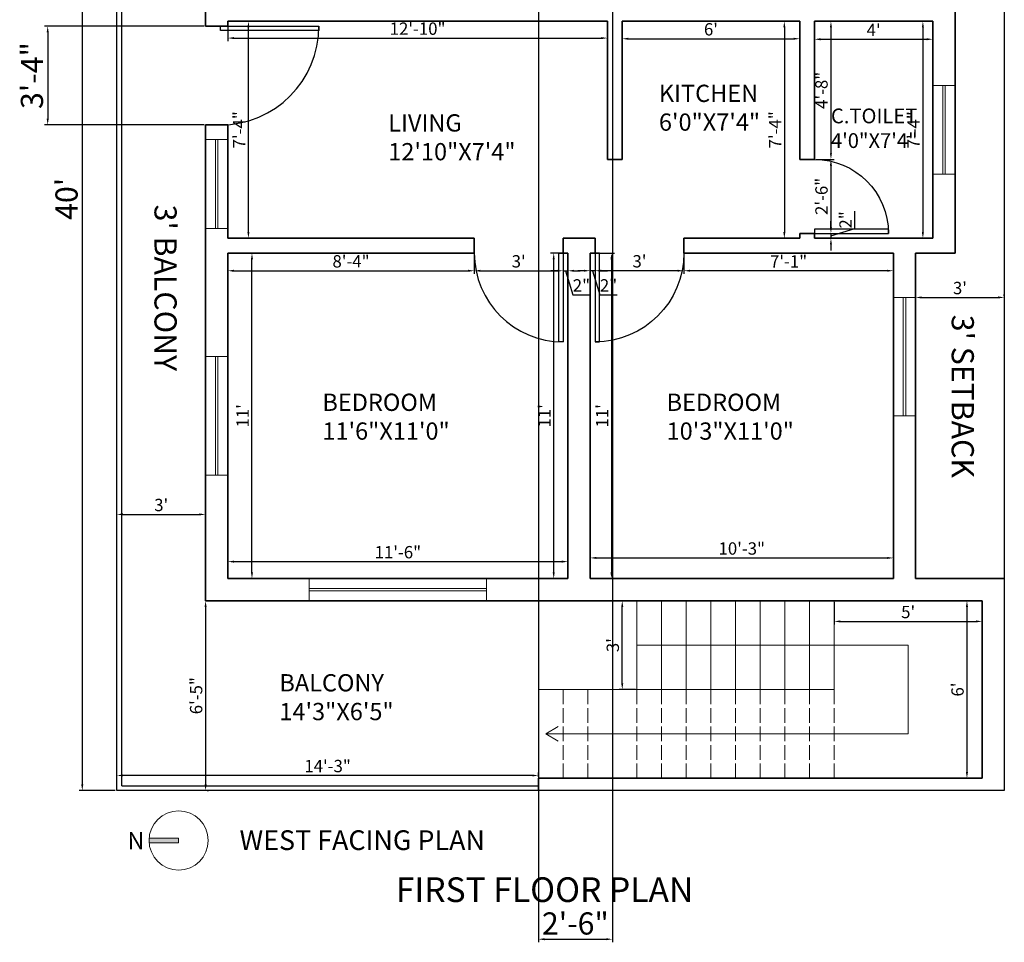
# Model space of a CAD drawing. Units: inches. Extents: x 2831 to 4250, y 1103 to 1797.
# Tile 14 of 15: x 3821 to 4220, y 1181 to 1555. Entities that reach past the tile are written whole.
import ezdxf

# ---------------------------------------------------------------- set-up
doc = ezdxf.new("R2010")
doc.units = ezdxf.units.IN
doc.linetypes.add('ACAD_ISO02W100', pattern=[15, 12, -3])
for name, color, linetype, lineweight in [('A-ANNO-DIMS', 2, 'Continuous', 18), ('A-ANNO-SYMB', 7, 'Continuous', 18), ('A-ANNO-TEXT', 7, 'Continuous', 18), ('A-ANNO-TITL', 7, 'Continuous', 25), ('A-AREA-IDEN', 7, 'Continuous', 18), ('A-DOOR', 4, 'Continuous', 25), ('A-FLOR-STRS', 7, 'Continuous', 18), ('A-FLOR-STRS-HIDN', 8, 'ACAD_ISO02W100', 18), ('A-FLOR-STRS-IDEN', 1, 'Continuous', 18), ('A-WALL', 7, 'Continuous', 35), ('C-PROP', 7, 'Continuous', 25), ('window', 130, 'Continuous', 18)]:
    doc.layers.add(name, color=color, linetype=linetype, lineweight=lineweight)
doc.styles.get("Standard").update_dxf_attribs({"font": 'arial.ttf'})
doc.dimstyles.new('ISO-25', dxfattribs={"dimtxt": 9, "dimasz": 2.5, "dimexe": 1.25, "dimexo": 0.625, "dimtad": 1, "dimdec": 1, "dimlunit": 3, "dimtxsty": 'Standard', "dimcen": 2.5, "dimadec": 0, "dimazin": 0, "dimtfac": 1, "dimtdec": 1, "dimtmove": 0, "dimatfit": 3, "dimfxl": 1, "dimarcsym": 0})

# ---------------------------------------------------------------- blocks, each defined once
blk = doc.blocks.new('*U2')
for p, q in [((0, 0), (0, -6)), ((40, 0), (40, -6))]:
    blk.add_line(p, q)
blk.add_lwpolyline([(0, 0), (0, 40), (1.75, 40), (1.75, 0)], close=True)
blk.add_arc((0, 0), 40, 0, 90)
blk = doc.blocks.new('*U3')
for p, q in [((0, 0), (0, -6)), ((36, 0), (36, -6))]:
    blk.add_line(p, q)
blk.add_lwpolyline([(0, 0), (0, 36), (1.75, 36), (1.75, 0)], close=True)
blk.add_arc((0, 0), 36, 0, 90)
blk = doc.blocks.new('*U4')
for p, q in [((0, 0), (0, -6)), ((30, 0), (30, -6))]:
    blk.add_line(p, q)
blk.add_lwpolyline([(0, 0), (0, 30), (1.75, 30), (1.75, 0)], close=True)
blk.add_arc((0, 0), 30, 0, 90)
blk = doc.blocks.new('*D29')
at = {"layer": 'A-ANNO-DIMS', "color": 0, "lineweight": -2, "transparency": 16777216}
for p, q in [((3859.76, 1722.51), (3845.12, 1722.51)), ((3846.37, 1720.01), (3846.37, 1245.01)), ((3859.76, 1242.51), (3845.12, 1242.51))]:
    blk.add_line(p, q, dxfattribs=at)
at = {"layer": 'A-ANNO-DIMS', "color": 0, "transparency": 16777216}
for points in [[(3845.95, 1720.01), (3846.79, 1720.01), (3846.37, 1722.51)], [(3845.95, 1245.01), (3846.79, 1245.01), (3846.37, 1242.51)]]:
    blk.add_solid(points, dxfattribs=at)
at = {"layer": 'Defpoints', "color": 0, "transparency": 16777216}
for p in [(3860.39, 1722.51), (3846.37, 1242.51), (3860.39, 1242.51)]:
    blk.add_point(p, dxfattribs=at)
at = {"layer": 'A-ANNO-DIMS', "color": 0, "transparency": 16777216, "insert": (3841.15, 1482.51), "char_height": 9, "attachment_point": 5, "rotation": 90}
blk.add_mtext("40'", dxfattribs=at)
blk = doc.blocks.new('*D39')
at = {"layer": 'A-ANNO-DIMS', "color": 0, "lineweight": -2, "transparency": 16777216}
for p, q in [((3905.39, 1553.89), (3905.39, 1546.45)), ((4059.39, 1553.89), (4059.39, 1546.45)), ((3907.89, 1547.7), (4056.89, 1547.7))]:
    blk.add_line(p, q, dxfattribs=at)
at = {"layer": 'A-ANNO-DIMS', "color": 0, "transparency": 16777216}
for points in [[(3907.89, 1548.12), (3907.89, 1547.29), (3905.39, 1547.7)], [(4056.89, 1548.12), (4056.89, 1547.29), (4059.39, 1547.7)]]:
    blk.add_solid(points, dxfattribs=at)
at = {"layer": 'Defpoints', "color": 0, "transparency": 16777216}
for p in [(3905.39, 1554.51), (4059.39, 1554.51), (4059.39, 1547.7)]:
    blk.add_point(p, dxfattribs=at)
at = {"layer": 'A-ANNO-DIMS', "color": 0, "transparency": 16777216, "insert": (3982.39, 1550.88), "char_height": 5, "attachment_point": 5}
blk.add_mtext('12\'-10"', dxfattribs=at)
blk = doc.blocks.new('*D40')
at = {"layer": 'A-ANNO-DIMS', "color": 0, "lineweight": -2, "transparency": 16777216}
for p, q in [((3906.01, 1554.51), (3915.02, 1554.51)), ((3913.77, 1469.01), (3913.77, 1552.01)), ((3906.01, 1466.51), (3915.02, 1466.51))]:
    blk.add_line(p, q, dxfattribs=at)
at = {"layer": 'A-ANNO-DIMS', "color": 0, "transparency": 16777216}
for points in [[(3913.35, 1552.01), (3914.18, 1552.01), (3913.77, 1554.51)], [(3913.35, 1469.01), (3914.18, 1469.01), (3913.77, 1466.51)]]:
    blk.add_solid(points, dxfattribs=at)
at = {"layer": 'Defpoints', "color": 0, "transparency": 16777216}
for p in [(3905.39, 1554.51), (3913.77, 1554.51), (3905.39, 1466.51)]:
    blk.add_point(p, dxfattribs=at)
at = {"layer": 'A-ANNO-DIMS', "color": 0, "transparency": 16777216, "insert": (3910.64, 1510.51), "char_height": 5, "attachment_point": 5, "rotation": 90}
blk.add_mtext('7\'-4"', dxfattribs=at)
blk = doc.blocks.new('*D41')
at = {"layer": 'A-ANNO-DIMS', "color": 0, "lineweight": -2, "transparency": 16777216}
for p, q in [((4065.39, 1553.89), (4065.39, 1546.18)), ((4137.39, 1553.89), (4137.39, 1546.18)), ((4067.89, 1547.43), (4134.89, 1547.43))]:
    blk.add_line(p, q, dxfattribs=at)
at = {"layer": 'A-ANNO-DIMS', "color": 0, "transparency": 16777216}
for points in [[(4067.89, 1547.85), (4067.89, 1547.02), (4065.39, 1547.43)], [(4134.89, 1547.85), (4134.89, 1547.02), (4137.39, 1547.43)]]:
    blk.add_solid(points, dxfattribs=at)
at = {"layer": 'Defpoints', "color": 0, "transparency": 16777216}
for p in [(4065.39, 1554.51), (4137.39, 1554.51), (4137.39, 1547.43)]:
    blk.add_point(p, dxfattribs=at)
at = {"layer": 'A-ANNO-DIMS', "color": 0, "transparency": 16777216, "insert": (4101.39, 1550.61), "char_height": 5, "attachment_point": 5}
blk.add_mtext("6'", dxfattribs=at)
blk = doc.blocks.new('*D42')
at = {"layer": 'A-ANNO-DIMS', "color": 0, "lineweight": -2, "transparency": 16777216}
for p, q in [((4143.39, 1553.89), (4143.39, 1545.97)), ((4191.39, 1553.89), (4191.39, 1545.97)), ((4145.89, 1547.22), (4188.89, 1547.22))]:
    blk.add_line(p, q, dxfattribs=at)
at = {"layer": 'A-ANNO-DIMS', "color": 0, "transparency": 16777216}
for points in [[(4145.89, 1547.64), (4145.89, 1546.8), (4143.39, 1547.22)], [(4188.89, 1547.64), (4188.89, 1546.8), (4191.39, 1547.22)]]:
    blk.add_solid(points, dxfattribs=at)
at = {"layer": 'Defpoints', "color": 0, "transparency": 16777216}
for p in [(4143.39, 1554.51), (4191.39, 1554.51), (4191.39, 1547.22)]:
    blk.add_point(p, dxfattribs=at)
at = {"layer": 'A-ANNO-DIMS', "color": 0, "transparency": 16777216, "insert": (4167.39, 1550.34), "char_height": 5, "attachment_point": 5}
blk.add_mtext("4'", dxfattribs=at)
blk = doc.blocks.new('*D43')
at = {"layer": 'A-ANNO-DIMS', "color": 0, "lineweight": -2, "transparency": 16777216}
for p, q in [((4190.76, 1554.51), (4186.11, 1554.51)), ((4187.36, 1552.01), (4187.36, 1469.01)), ((4190.76, 1466.51), (4186.11, 1466.51))]:
    blk.add_line(p, q, dxfattribs=at)
at = {"layer": 'A-ANNO-DIMS', "color": 0, "transparency": 16777216}
for points in [[(4186.94, 1552.01), (4187.77, 1552.01), (4187.36, 1554.51)], [(4186.94, 1469.01), (4187.77, 1469.01), (4187.36, 1466.51)]]:
    blk.add_solid(points, dxfattribs=at)
at = {"layer": 'Defpoints', "color": 0, "transparency": 16777216}
for p in [(4191.39, 1554.51), (4187.36, 1466.51), (4191.39, 1466.51)]:
    blk.add_point(p, dxfattribs=at)
at = {"layer": 'A-ANNO-DIMS', "color": 0, "transparency": 16777216, "insert": (4184.23, 1510.51), "char_height": 5, "attachment_point": 5, "rotation": 90}
blk.add_mtext('7\'-4"', dxfattribs=at)
blk = doc.blocks.new('*D44')
at = {"layer": 'A-ANNO-DIMS', "color": 0, "lineweight": -2, "transparency": 16777216}
for p, q in [((4144.01, 1554.51), (4151.31, 1554.51)), ((4150.06, 1552.01), (4150.06, 1501.01)), ((4144.01, 1498.51), (4151.31, 1498.51))]:
    blk.add_line(p, q, dxfattribs=at)
at = {"layer": 'A-ANNO-DIMS', "color": 0, "transparency": 16777216}
for points in [[(4149.64, 1552.01), (4150.47, 1552.01), (4150.06, 1554.51)], [(4149.64, 1501.01), (4150.47, 1501.01), (4150.06, 1498.51)]]:
    blk.add_solid(points, dxfattribs=at)
at = {"layer": 'Defpoints', "color": 0, "transparency": 16777216}
for p in [(4143.39, 1554.51), (4143.39, 1498.51), (4150.06, 1498.51)]:
    blk.add_point(p, dxfattribs=at)
at = {"layer": 'A-ANNO-DIMS', "color": 0, "transparency": 16777216, "insert": (4146.88, 1526.51), "char_height": 5, "attachment_point": 5, "rotation": 90}
blk.add_mtext('4\'-8"', dxfattribs=at)
blk = doc.blocks.new('*D45')
at = {"layer": 'A-ANNO-DIMS', "color": 0, "lineweight": -2, "transparency": 16777216}
for p, q in [((4144.01, 1498.51), (4151.31, 1498.51)), ((4150.06, 1496.01), (4150.06, 1471.01)), ((4144.01, 1468.51), (4151.31, 1468.51))]:
    blk.add_line(p, q, dxfattribs=at)
at = {"layer": 'A-ANNO-DIMS', "color": 0, "transparency": 16777216}
for points in [[(4149.64, 1496.01), (4150.47, 1496.01), (4150.06, 1498.51)], [(4149.64, 1471.01), (4150.47, 1471.01), (4150.06, 1468.51)]]:
    blk.add_solid(points, dxfattribs=at)
at = {"layer": 'Defpoints', "color": 0, "transparency": 16777216}
for p in [(4143.39, 1498.51), (4143.39, 1468.51), (4150.06, 1468.51)]:
    blk.add_point(p, dxfattribs=at)
at = {"layer": 'A-ANNO-DIMS', "color": 0, "transparency": 16777216, "insert": (4146.88, 1483.51), "char_height": 5, "attachment_point": 5, "rotation": 90}
blk.add_mtext('2\'-6"', dxfattribs=at)
blk = doc.blocks.new('*D46')
at = {"layer": 'A-ANNO-DIMS', "color": 0, "lineweight": -2, "transparency": 16777216}
for p, q in [((4159.78, 1470.43), (4159.78, 1477.51)), ((4150.06, 1471.01), (4150.06, 1473.51)), ((4150.06, 1467.51), (4159.78, 1470.43)), ((4144.01, 1468.51), (4151.31, 1468.51)), ((4144.01, 1466.51), (4151.31, 1466.51)), ((4150.06, 1468.51), (4150.06, 1466.51)), ((4150.06, 1468.51), (4150.06, 1466.51)), ((4150.06, 1464.01), (4150.06, 1461.51))]:
    blk.add_line(p, q, dxfattribs=at)
at = {"layer": 'A-ANNO-DIMS', "color": 0, "transparency": 16777216}
for points in [[(4149.64, 1471.01), (4150.47, 1471.01), (4150.06, 1468.51)], [(4149.64, 1464.01), (4150.47, 1464.01), (4150.06, 1466.51)]]:
    blk.add_solid(points, dxfattribs=at)
at = {"layer": 'Defpoints', "color": 0, "transparency": 16777216}
for p in [(4143.39, 1468.51), (4143.39, 1466.51), (4150.06, 1466.51)]:
    blk.add_point(p, dxfattribs=at)
at = {"layer": 'A-ANNO-DIMS', "color": 0, "transparency": 16777216, "insert": (4156.64, 1473.97), "char_height": 5, "attachment_point": 5, "rotation": 90}
blk.add_mtext('2"', dxfattribs=at)
blk = doc.blocks.new('*D47')
at = {"layer": 'A-ANNO-DIMS', "color": 0, "lineweight": -2, "transparency": 16777216}
for p, q in [((4184.39, 1443.14), (4184.39, 1443.76)), ((4186.89, 1442.51), (4217.89, 1442.51)), ((4220.39, 1443.14), (4220.39, 1443.76))]:
    blk.add_line(p, q, dxfattribs=at)
at = {"layer": 'A-ANNO-DIMS', "color": 0, "transparency": 16777216}
for points in [[(4186.89, 1442.93), (4186.89, 1442.1), (4184.39, 1442.51)], [(4217.89, 1442.93), (4217.89, 1442.1), (4220.39, 1442.51)]]:
    blk.add_solid(points, dxfattribs=at)
at = {"layer": 'Defpoints', "color": 0, "transparency": 16777216}
for p in [(4184.39, 1442.51), (4220.39, 1442.51), (4220.39, 1442.51)]:
    blk.add_point(p, dxfattribs=at)
at = {"layer": 'A-ANNO-DIMS', "color": 0, "transparency": 16777216, "insert": (4202.39, 1445.69), "char_height": 5, "attachment_point": 5}
blk.add_mtext("3'", dxfattribs=at)
blk = doc.blocks.new('*D48')
at = {"layer": 'A-ANNO-DIMS', "color": 0, "lineweight": -2, "transparency": 16777216}
for p, q in [((4090.39, 1459.89), (4090.39, 1452.11)), ((4175.39, 1459.89), (4175.39, 1452.11)), ((4172.89, 1453.36), (4092.89, 1453.36))]:
    blk.add_line(p, q, dxfattribs=at)
at = {"layer": 'A-ANNO-DIMS', "color": 0, "transparency": 16777216}
for points in [[(4092.89, 1453.77), (4092.89, 1452.94), (4090.39, 1453.36)], [(4172.89, 1453.77), (4172.89, 1452.94), (4175.39, 1453.36)]]:
    blk.add_solid(points, dxfattribs=at)
at = {"layer": 'Defpoints', "color": 0, "transparency": 16777216}
for p in [(4090.39, 1460.51), (4175.39, 1460.51), (4090.39, 1453.36)]:
    blk.add_point(p, dxfattribs=at)
at = {"layer": 'A-ANNO-DIMS', "color": 0, "transparency": 16777216, "insert": (4132.89, 1456.49), "char_height": 5, "attachment_point": 5}
blk.add_mtext('7\'-1"', dxfattribs=at)
blk = doc.blocks.new('*D49')
at = {"layer": 'A-ANNO-DIMS', "color": 0, "lineweight": -2, "transparency": 16777216}
for p, q in [((4054.39, 1459.89), (4054.39, 1452.11)), ((4090.39, 1459.89), (4090.39, 1452.11)), ((4087.89, 1453.36), (4056.89, 1453.36))]:
    blk.add_line(p, q, dxfattribs=at)
at = {"layer": 'A-ANNO-DIMS', "color": 0, "transparency": 16777216}
for points in [[(4056.89, 1453.77), (4056.89, 1452.94), (4054.39, 1453.36)], [(4087.89, 1453.77), (4087.89, 1452.94), (4090.39, 1453.36)]]:
    blk.add_solid(points, dxfattribs=at)
at = {"layer": 'Defpoints', "color": 0, "transparency": 16777216}
for p in [(4054.39, 1460.51), (4090.39, 1460.51), (4054.39, 1453.36)]:
    blk.add_point(p, dxfattribs=at)
at = {"layer": 'A-ANNO-DIMS', "color": 0, "transparency": 16777216, "insert": (4072.39, 1456.54), "char_height": 5, "attachment_point": 5}
blk.add_mtext("3'", dxfattribs=at)
blk = doc.blocks.new('*D50')
at = {"layer": 'A-ANNO-DIMS', "color": 0, "lineweight": -2, "transparency": 16777216}
for p, q in [((4052.39, 1459.89), (4052.39, 1452.11)), ((4054.39, 1459.89), (4054.39, 1452.11)), ((4049.89, 1453.36), (4047.39, 1453.36)), ((4054.39, 1453.36), (4052.39, 1453.36)), ((4054.39, 1453.36), (4052.39, 1453.36)), ((4053.39, 1453.36), (4056.3, 1443.64)), ((4056.89, 1453.36), (4059.39, 1453.36)), ((4056.3, 1443.64), (4063.39, 1443.64))]:
    blk.add_line(p, q, dxfattribs=at)
at = {"layer": 'A-ANNO-DIMS', "color": 0, "transparency": 16777216}
for points in [[(4049.89, 1453.77), (4049.89, 1452.94), (4052.39, 1453.36)], [(4056.89, 1453.77), (4056.89, 1452.94), (4054.39, 1453.36)]]:
    blk.add_solid(points, dxfattribs=at)
at = {"layer": 'Defpoints', "color": 0, "transparency": 16777216}
for p in [(4052.39, 1460.51), (4054.39, 1460.51), (4052.39, 1453.36)]:
    blk.add_point(p, dxfattribs=at)
at = {"layer": 'A-ANNO-DIMS', "color": 0, "transparency": 16777216, "insert": (4059.85, 1446.77), "char_height": 5, "attachment_point": 5}
blk.add_mtext('2"', dxfattribs=at)
blk = doc.blocks.new('*D51')
at = {"layer": 'A-ANNO-DIMS', "color": 0, "lineweight": -2, "transparency": 16777216}
for p, q in [((4053.01, 1460.51), (4062.29, 1460.51)), ((4061.04, 1458.01), (4061.04, 1331.01)), ((4053.01, 1328.51), (4062.29, 1328.51))]:
    blk.add_line(p, q, dxfattribs=at)
at = {"layer": 'A-ANNO-DIMS', "color": 0, "transparency": 16777216}
for points in [[(4060.63, 1458.01), (4061.46, 1458.01), (4061.04, 1460.51)], [(4060.63, 1331.01), (4061.46, 1331.01), (4061.04, 1328.51)]]:
    blk.add_solid(points, dxfattribs=at)
at = {"layer": 'Defpoints', "color": 0, "transparency": 16777216}
for p in [(4052.39, 1460.51), (4052.39, 1328.51), (4061.04, 1328.51)]:
    blk.add_point(p, dxfattribs=at)
at = {"layer": 'A-ANNO-DIMS', "color": 0, "transparency": 16777216, "insert": (4057.91, 1394.51), "char_height": 5, "attachment_point": 5, "rotation": 90}
blk.add_mtext("11'", dxfattribs=at)
blk = doc.blocks.new('*D52')
at = {"layer": 'A-ANNO-DIMS', "color": 0, "lineweight": -2, "transparency": 16777216}
for p, q in [((4052.39, 1329.14), (4052.39, 1338.13)), ((4175.39, 1329.14), (4175.39, 1338.13)), ((4054.89, 1336.88), (4172.89, 1336.88))]:
    blk.add_line(p, q, dxfattribs=at)
at = {"layer": 'A-ANNO-DIMS', "color": 0, "transparency": 16777216}
for points in [[(4054.89, 1337.3), (4054.89, 1336.47), (4052.39, 1336.88)], [(4172.89, 1337.3), (4172.89, 1336.47), (4175.39, 1336.88)]]:
    blk.add_solid(points, dxfattribs=at)
at = {"layer": 'Defpoints', "color": 0, "transparency": 16777216}
for p in [(4175.39, 1336.88), (4052.39, 1328.51), (4175.39, 1328.51)]:
    blk.add_point(p, dxfattribs=at)
at = {"layer": 'A-ANNO-DIMS', "color": 0, "transparency": 16777216, "insert": (4113.89, 1340.06), "char_height": 5, "attachment_point": 5}
blk.add_mtext('10\'-3"', dxfattribs=at)
blk = doc.blocks.new('*D53')
at = {"layer": 'A-ANNO-DIMS', "color": 0, "lineweight": -2, "transparency": 16777216}
for p, q in [((3905.39, 1329.14), (3905.39, 1336.63)), ((3907.89, 1335.38), (4040.89, 1335.38)), ((4043.39, 1329.14), (4043.39, 1336.63))]:
    blk.add_line(p, q, dxfattribs=at)
at = {"layer": 'A-ANNO-DIMS', "color": 0, "transparency": 16777216}
for points in [[(3907.89, 1335.8), (3907.89, 1334.96), (3905.39, 1335.38)], [(4040.89, 1335.8), (4040.89, 1334.96), (4043.39, 1335.38)]]:
    blk.add_solid(points, dxfattribs=at)
at = {"layer": 'Defpoints', "color": 0, "transparency": 16777216}
for p in [(4043.39, 1335.38), (3905.39, 1328.51), (4043.39, 1328.51)]:
    blk.add_point(p, dxfattribs=at)
at = {"layer": 'A-ANNO-DIMS', "color": 0, "transparency": 16777216, "insert": (3974.39, 1338.56), "char_height": 5, "attachment_point": 5}
blk.add_mtext('11\'-6"', dxfattribs=at)
blk = doc.blocks.new('*D54')
at = {"layer": 'A-ANNO-DIMS', "color": 0, "lineweight": -2, "transparency": 16777216}
for p, q in [((4042.76, 1460.51), (4036.36, 1460.51)), ((4037.61, 1331.01), (4037.61, 1458.01)), ((4042.76, 1328.51), (4036.36, 1328.51))]:
    blk.add_line(p, q, dxfattribs=at)
at = {"layer": 'A-ANNO-DIMS', "color": 0, "transparency": 16777216}
for points in [[(4037.19, 1458.01), (4038.02, 1458.01), (4037.61, 1460.51)], [(4037.19, 1331.01), (4038.02, 1331.01), (4037.61, 1328.51)]]:
    blk.add_solid(points, dxfattribs=at)
at = {"layer": 'Defpoints', "color": 0, "transparency": 16777216}
for p in [(4037.61, 1460.51), (4043.39, 1460.51), (4043.39, 1328.51)]:
    blk.add_point(p, dxfattribs=at)
at = {"layer": 'A-ANNO-DIMS', "color": 0, "transparency": 16777216, "insert": (4034.47, 1394.51), "char_height": 5, "attachment_point": 5, "rotation": 90}
blk.add_mtext("11'", dxfattribs=at)
blk = doc.blocks.new('*D55')
at = {"layer": 'A-ANNO-DIMS', "color": 0, "lineweight": -2, "transparency": 16777216}
for p, q in [((3906.01, 1460.51), (3916.46, 1460.51)), ((3915.21, 1331.01), (3915.21, 1458.01)), ((3906.01, 1328.51), (3916.46, 1328.51))]:
    blk.add_line(p, q, dxfattribs=at)
at = {"layer": 'A-ANNO-DIMS', "color": 0, "transparency": 16777216}
for points in [[(3914.79, 1458.01), (3915.62, 1458.01), (3915.21, 1460.51)], [(3914.79, 1331.01), (3915.62, 1331.01), (3915.21, 1328.51)]]:
    blk.add_solid(points, dxfattribs=at)
at = {"layer": 'Defpoints', "color": 0, "transparency": 16777216}
for p in [(3905.39, 1460.51), (3915.21, 1460.51), (3905.39, 1328.51)]:
    blk.add_point(p, dxfattribs=at)
at = {"layer": 'A-ANNO-DIMS', "color": 0, "transparency": 16777216, "insert": (3912.07, 1394.51), "char_height": 5, "attachment_point": 5, "rotation": 90}
blk.add_mtext("11'", dxfattribs=at)
blk = doc.blocks.new('*D56')
at = {"layer": 'A-ANNO-DIMS', "color": 0, "lineweight": -2, "transparency": 16777216}
for p, q in [((3905.39, 1459.89), (3905.39, 1452.09)), ((4005.39, 1459.89), (4005.39, 1452.09)), ((3907.89, 1453.34), (4002.89, 1453.34))]:
    blk.add_line(p, q, dxfattribs=at)
at = {"layer": 'A-ANNO-DIMS', "color": 0, "transparency": 16777216}
for points in [[(3907.89, 1453.75), (3907.89, 1452.92), (3905.39, 1453.34)], [(4002.89, 1453.75), (4002.89, 1452.92), (4005.39, 1453.34)]]:
    blk.add_solid(points, dxfattribs=at)
at = {"layer": 'Defpoints', "color": 0, "transparency": 16777216}
for p in [(3905.39, 1460.51), (4005.39, 1460.51), (4005.39, 1453.34)]:
    blk.add_point(p, dxfattribs=at)
at = {"layer": 'A-ANNO-DIMS', "color": 0, "transparency": 16777216, "insert": (3955.39, 1456.52), "char_height": 5, "attachment_point": 5}
blk.add_mtext('8\'-4"', dxfattribs=at)
blk = doc.blocks.new('*D57')
at = {"layer": 'A-ANNO-DIMS', "color": 0, "lineweight": -2, "transparency": 16777216}
for p, q in [((4005.39, 1459.89), (4005.39, 1452.09)), ((4041.39, 1459.89), (4041.39, 1452.09)), ((4007.89, 1453.34), (4038.89, 1453.34))]:
    blk.add_line(p, q, dxfattribs=at)
at = {"layer": 'A-ANNO-DIMS', "color": 0, "transparency": 16777216}
for points in [[(4007.89, 1453.75), (4007.89, 1452.92), (4005.39, 1453.34)], [(4038.89, 1453.75), (4038.89, 1452.92), (4041.39, 1453.34)]]:
    blk.add_solid(points, dxfattribs=at)
at = {"layer": 'Defpoints', "color": 0, "transparency": 16777216}
for p in [(4005.39, 1460.51), (4041.39, 1460.51), (4041.39, 1453.34)]:
    blk.add_point(p, dxfattribs=at)
at = {"layer": 'A-ANNO-DIMS', "color": 0, "transparency": 16777216, "insert": (4023.39, 1456.52), "char_height": 5, "attachment_point": 5}
blk.add_mtext("3'", dxfattribs=at)
blk = doc.blocks.new('*D58')
at = {"layer": 'A-ANNO-DIMS', "color": 0, "lineweight": -2, "transparency": 16777216}
for p, q in [((4041.39, 1459.89), (4041.39, 1452.09)), ((4043.39, 1459.89), (4043.39, 1452.09)), ((4038.89, 1453.34), (4036.39, 1453.34)), ((4041.39, 1453.34), (4043.39, 1453.34)), ((4041.39, 1453.34), (4043.39, 1453.34)), ((4042.39, 1453.34), (4045.3, 1443.62)), ((4045.89, 1453.34), (4048.39, 1453.34)), ((4045.3, 1443.62), (4052.39, 1443.62))]:
    blk.add_line(p, q, dxfattribs=at)
at = {"layer": 'A-ANNO-DIMS', "color": 0, "transparency": 16777216}
for points in [[(4038.89, 1453.75), (4038.89, 1452.92), (4041.39, 1453.34)], [(4045.89, 1453.75), (4045.89, 1452.92), (4043.39, 1453.34)]]:
    blk.add_solid(points, dxfattribs=at)
at = {"layer": 'Defpoints', "color": 0, "transparency": 16777216}
for p in [(4041.39, 1460.51), (4043.39, 1460.51), (4043.39, 1453.34)]:
    blk.add_point(p, dxfattribs=at)
at = {"layer": 'A-ANNO-DIMS', "color": 0, "transparency": 16777216, "insert": (4048.85, 1446.76), "char_height": 5, "attachment_point": 5}
blk.add_mtext('2"', dxfattribs=at)
blk = doc.blocks.new('*D59')
at = {"layer": 'A-ANNO-DIMS', "color": 0, "lineweight": -2, "transparency": 16777216}
for p, q in [((4136.76, 1554.51), (4129.91, 1554.51)), ((4131.16, 1552.01), (4131.16, 1469.01)), ((4136.76, 1466.51), (4129.91, 1466.51))]:
    blk.add_line(p, q, dxfattribs=at)
at = {"layer": 'A-ANNO-DIMS', "color": 0, "transparency": 16777216}
for points in [[(4130.75, 1552.01), (4131.58, 1552.01), (4131.16, 1554.51)], [(4130.75, 1469.01), (4131.58, 1469.01), (4131.16, 1466.51)]]:
    blk.add_solid(points, dxfattribs=at)
at = {"layer": 'Defpoints', "color": 0, "transparency": 16777216}
for p in [(4137.39, 1554.51), (4131.16, 1466.51), (4137.39, 1466.51)]:
    blk.add_point(p, dxfattribs=at)
at = {"layer": 'A-ANNO-DIMS', "color": 0, "transparency": 16777216, "insert": (4128.04, 1510.51), "char_height": 5, "attachment_point": 5, "rotation": 90}
blk.add_mtext('7\'-4"', dxfattribs=at)
blk = doc.blocks.new('*D60')
at = {"layer": 'A-ANNO-DIMS', "color": 0, "lineweight": -2, "transparency": 16777216}
for p, q in [((3897.01, 1319.51), (3897.64, 1319.51)), ((3896.39, 1317.01), (3896.39, 1245.01)), ((3897.01, 1242.51), (3897.64, 1242.51))]:
    blk.add_line(p, q, dxfattribs=at)
at = {"layer": 'A-ANNO-DIMS', "color": 0, "transparency": 16777216}
for points in [[(3895.97, 1317.01), (3896.81, 1317.01), (3896.39, 1319.51)], [(3895.97, 1245.01), (3896.81, 1245.01), (3896.39, 1242.51)]]:
    blk.add_solid(points, dxfattribs=at)
at = {"layer": 'Defpoints', "color": 0, "transparency": 16777216}
for p in [(3896.39, 1319.51), (3896.39, 1242.51), (3896.39, 1242.51)]:
    blk.add_point(p, dxfattribs=at)
at = {"layer": 'A-ANNO-DIMS', "color": 0, "transparency": 16777216, "insert": (3893.21, 1281.01), "char_height": 5, "attachment_point": 5, "rotation": 90}
blk.add_mtext('6\'-5"', dxfattribs=at)
blk = doc.blocks.new('*D61')
at = {"layer": 'A-ANNO-DIMS', "color": 0, "lineweight": -2, "transparency": 16777216}
for p, q in [((3860.39, 1248.14), (3860.39, 1249.9)), ((4028.89, 1248.65), (3862.89, 1248.65)), ((4031.39, 1248.14), (4031.39, 1249.9))]:
    blk.add_line(p, q, dxfattribs=at)
at = {"layer": 'A-ANNO-DIMS', "color": 0, "transparency": 16777216}
for points in [[(3862.89, 1249.07), (3862.89, 1248.24), (3860.39, 1248.65)], [(4028.89, 1249.07), (4028.89, 1248.24), (4031.39, 1248.65)]]:
    blk.add_solid(points, dxfattribs=at)
at = {"layer": 'Defpoints', "color": 0, "transparency": 16777216}
for p in [(3860.39, 1248.65), (3860.39, 1247.51), (4031.39, 1247.51)]:
    blk.add_point(p, dxfattribs=at)
at = {"layer": 'A-ANNO-DIMS', "color": 0, "transparency": 16777216, "insert": (3945.89, 1251.83), "char_height": 5, "attachment_point": 5}
blk.add_mtext('14\'-3"', dxfattribs=at)
blk = doc.blocks.new('*D62')
at = {"layer": 'A-ANNO-DIMS', "color": 0, "lineweight": -2, "transparency": 16777216}
for p, q in [((4070.76, 1319.51), (4064.16, 1319.51)), ((4065.41, 1286.01), (4065.41, 1317.01)), ((4070.76, 1283.51), (4064.16, 1283.51))]:
    blk.add_line(p, q, dxfattribs=at)
at = {"layer": 'A-ANNO-DIMS', "color": 0, "transparency": 16777216}
for points in [[(4064.99, 1317.01), (4065.82, 1317.01), (4065.41, 1319.51)], [(4064.99, 1286.01), (4065.82, 1286.01), (4065.41, 1283.51)]]:
    blk.add_solid(points, dxfattribs=at)
at = {"layer": 'Defpoints', "color": 0, "transparency": 16777216}
for p in [(4065.41, 1319.51), (4071.39, 1319.51), (4071.39, 1283.51)]:
    blk.add_point(p, dxfattribs=at)
at = {"layer": 'A-ANNO-DIMS', "color": 0, "transparency": 16777216, "insert": (4062.23, 1301.51), "char_height": 5, "attachment_point": 5, "rotation": 90}
blk.add_mtext("3'", dxfattribs=at)
blk = doc.blocks.new('*D63')
at = {"layer": 'A-ANNO-DIMS', "color": 0, "lineweight": -2, "transparency": 16777216}
for p, q in [((4151.39, 1318.89), (4151.39, 1309.88)), ((4211.39, 1318.89), (4211.39, 1309.88)), ((4153.89, 1311.13), (4208.89, 1311.13))]:
    blk.add_line(p, q, dxfattribs=at)
at = {"layer": 'A-ANNO-DIMS', "color": 0, "transparency": 16777216}
for points in [[(4153.89, 1311.55), (4153.89, 1310.72), (4151.39, 1311.13)], [(4208.89, 1311.55), (4208.89, 1310.72), (4211.39, 1311.13)]]:
    blk.add_solid(points, dxfattribs=at)
at = {"layer": 'Defpoints', "color": 0, "transparency": 16777216}
for p in [(4151.39, 1319.51), (4211.39, 1319.51), (4211.39, 1311.13)]:
    blk.add_point(p, dxfattribs=at)
at = {"layer": 'A-ANNO-DIMS', "color": 0, "transparency": 16777216, "insert": (4181.39, 1314.3), "char_height": 5, "attachment_point": 5}
blk.add_mtext("5'", dxfattribs=at)
blk = doc.blocks.new('*D64')
at = {"layer": 'A-ANNO-DIMS', "color": 0, "lineweight": -2, "transparency": 16777216}
for p, q in [((4210.76, 1319.51), (4203.98, 1319.51)), ((4205.23, 1317.01), (4205.23, 1250.01)), ((4210.76, 1247.51), (4203.98, 1247.51))]:
    blk.add_line(p, q, dxfattribs=at)
at = {"layer": 'A-ANNO-DIMS', "color": 0, "transparency": 16777216}
for points in [[(4204.82, 1317.01), (4205.65, 1317.01), (4205.23, 1319.51)], [(4204.82, 1250.01), (4205.65, 1250.01), (4205.23, 1247.51)]]:
    blk.add_solid(points, dxfattribs=at)
at = {"layer": 'Defpoints', "color": 0, "transparency": 16777216}
for p in [(4211.39, 1319.51), (4205.23, 1247.51), (4211.39, 1247.51)]:
    blk.add_point(p, dxfattribs=at)
at = {"layer": 'A-ANNO-DIMS', "color": 0, "transparency": 16777216, "insert": (4202.06, 1283.51), "char_height": 5, "attachment_point": 5, "rotation": 90}
blk.add_mtext("6'", dxfattribs=at)
blk = doc.blocks.new('*D67')
at = {"layer": 'A-ANNO-DIMS', "color": 0, "lineweight": -2, "transparency": 16777216}
for p, q in [((3860.39, 1355.15), (3860.39, 1355.77)), ((3862.89, 1354.52), (3893.89, 1354.52)), ((3896.39, 1355.15), (3896.39, 1355.77))]:
    blk.add_line(p, q, dxfattribs=at)
at = {"layer": 'A-ANNO-DIMS', "color": 0, "transparency": 16777216}
for points in [[(3862.89, 1354.94), (3862.89, 1354.11), (3860.39, 1354.52)], [(3893.89, 1354.94), (3893.89, 1354.11), (3896.39, 1354.52)]]:
    blk.add_solid(points, dxfattribs=at)
at = {"layer": 'Defpoints', "color": 0, "transparency": 16777216}
for p in [(3860.39, 1354.52), (3896.39, 1354.52), (3896.39, 1354.52)]:
    blk.add_point(p, dxfattribs=at)
at = {"layer": 'A-ANNO-DIMS', "color": 0, "transparency": 16777216, "insert": (3878.39, 1357.7), "char_height": 5, "attachment_point": 5}
blk.add_mtext("3'", dxfattribs=at)
blk = doc.blocks.new('WIN-36IN')
for p, q in [((0, 36), (9, 36)), ((4, 0), (4, 36)), ((5, 0), (5, 36)), ((0, 0), (9, 0))]:
    blk.add_line(p, q)
blk = doc.blocks.new('WIN-48IN')
for p, q in [((9, 48), (0, 48)), ((4, 0), (4, 48)), ((5, 0), (5, 48)), ((9, 0), (0, 0))]:
    blk.add_line(p, q)
blk = doc.blocks.new('WIN-72IN')
for p, q in [((0, 0), (0, 9)), ((72, 0), (72, 9)), ((0, 5), (72, 5)), ((0, 4), (72, 4))]:
    blk.add_line(p, q)
blk = doc.blocks.new('NORTH-MARK')
at = {"transparency": 33554687}
h = blk.add_hatch(color=256, dxfattribs=at)
h.dxf.hatch_style = 1
h.paths.add_polyline_path([(20.74, 13), (20.74, 11), (8.78, 11, -0.020861), (8.74, 12, -0.020861), (8.78, 13)])
for p, q in [((20.74, 13), (8.78, 13)), ((20.74, 11), (20.74, 13)), ((8.74, 11), (20.74, 11))]:
    blk.add_line(p, q)
blk.add_circle((20.74, 12), 12)
blk.add_text('N', height=6.9).set_placement((0, 8.47))
blk = doc.blocks.new('STAIR-TRAVEL-ARROW')
for points in [[(37, 39), (147, 39), (147, 3), (0, 3)], [(5, 0), (0, 3), (5, 6)]]:
    blk.add_lwpolyline(points)
blk = doc.blocks.new('*D100')
at = {"layer": 'A-ANNO-DIMS', "color": 0, "lineweight": -2, "transparency": 16777216}
for p, q in [((3895.76, 1552.51), (3831.09, 1552.51)), ((3832.34, 1550.01), (3832.34, 1515.01)), ((3895.76, 1512.51), (3831.09, 1512.51))]:
    blk.add_line(p, q, dxfattribs=at)
at = {"layer": 'A-ANNO-DIMS', "color": 0, "transparency": 16777216}
for points in [[(3831.92, 1550.01), (3832.76, 1550.01), (3832.34, 1552.51)], [(3831.92, 1515.01), (3832.76, 1515.01), (3832.34, 1512.51)]]:
    blk.add_solid(points, dxfattribs=at)
at = {"layer": 'Defpoints', "color": 0, "transparency": 16777216}
for p in [(3896.39, 1552.51), (3832.34, 1512.51), (3896.39, 1512.51)]:
    blk.add_point(p, dxfattribs=at)
at = {"layer": 'A-ANNO-DIMS', "color": 0, "transparency": 16777216, "insert": (3827.12, 1532.51), "char_height": 9, "attachment_point": 5, "rotation": 90}
blk.add_mtext('3\'-4"', dxfattribs=at)
blk = doc.blocks.new('*D101')
at = {"layer": 'A-ANNO-DIMS', "color": 0, "lineweight": -2, "transparency": 16777216}
for p, q in [((4031.39, 1601.89), (4031.39, 1181)), ((4061.39, 1601.89), (4061.39, 1181)), ((4033.89, 1182.25), (4058.89, 1182.25))]:
    blk.add_line(p, q, dxfattribs=at)
at = {"layer": 'A-ANNO-DIMS', "color": 0, "transparency": 16777216}
for points in [[(4033.89, 1182.67), (4033.89, 1181.83), (4031.39, 1182.25)], [(4058.89, 1182.67), (4058.89, 1181.83), (4061.39, 1182.25)]]:
    blk.add_solid(points, dxfattribs=at)
at = {"layer": 'Defpoints', "color": 0, "transparency": 16777216}
for p in [(4031.39, 1602.51), (4061.39, 1602.51), (4061.39, 1182.25)]:
    blk.add_point(p, dxfattribs=at)
at = {"layer": 'A-ANNO-DIMS', "color": 0, "transparency": 16777216, "insert": (4046.39, 1187.47), "char_height": 9, "attachment_point": 5}
blk.add_mtext('2\'-6"', dxfattribs=at)

msp = doc.modelspace()

# ---------------------------------------------------------------- linework, layer by layer
at = {"layer": 'A-FLOR-STRS'}
for p, q in [((4071.39, 1319.51), (4071.39, 1283.51)), ((4081.39, 1319.51), (4081.39, 1283.51)), ((4091.39, 1319.51), (4091.39, 1283.51)), ((4101.39, 1319.51), (4101.39, 1283.51)), ((4111.39, 1319.51), (4111.39, 1283.51)), ((4121.39, 1319.51), (4121.39, 1283.51)), ((4131.39, 1319.51), (4131.39, 1283.51)), ((4141.39, 1319.51), (4141.39, 1283.51)), ((4151.39, 1319.51), (4151.39, 1283.51)), ((4151.39, 1283.51), (4031.39, 1283.51))]:
    msp.add_line(p, q, dxfattribs=at)
at = {"layer": 'A-FLOR-STRS-HIDN', "ltscale": 0.5}
for p, q in [((4031.39, 1283.51), (4031.39, 1247.51)), ((4041.39, 1283.51), (4041.39, 1247.51)), ((4051.39, 1283.51), (4051.39, 1247.51)), ((4061.39, 1283.51), (4061.39, 1247.51)), ((4071.39, 1283.51), (4071.39, 1247.51)), ((4081.39, 1283.51), (4081.39, 1247.51)), ((4091.39, 1283.51), (4091.39, 1247.51)), ((4101.39, 1283.51), (4101.39, 1247.51)), ((4111.39, 1283.51), (4111.39, 1247.51)), ((4121.39, 1283.51), (4121.39, 1247.51)), ((4131.39, 1283.51), (4131.39, 1247.51)), ((4141.39, 1283.51), (4141.39, 1247.51)), ((4151.39, 1283.51), (4151.39, 1247.51))]:
    msp.add_line(p, q, dxfattribs=at)
at = {"layer": 'A-WALL'}
for p, q in [((3896.39, 1552.51), (3896.39, 1562.51)), ((4200.39, 1460.51), (4200.39, 1560.51)), ((3905.39, 1554.51), (4059.39, 1554.51)), ((3905.39, 1552.51), (3905.39, 1554.51)), ((4059.39, 1498.51), (4059.39, 1554.51)), ((4065.39, 1554.51), (4137.39, 1554.51)), ((4065.39, 1498.51), (4065.39, 1554.51)), ((4137.39, 1498.51), (4137.39, 1554.51)), ((4143.39, 1554.51), (4191.39, 1554.51)), ((4143.39, 1498.51), (4143.39, 1554.51)), ((4191.39, 1466.51), (4191.39, 1554.51)), ((3896.39, 1552.51), (3905.39, 1552.51)), ((3896.39, 1512.51), (3905.39, 1512.51)), ((3896.39, 1319.51), (3896.39, 1512.51)), ((3905.39, 1466.51), (3905.39, 1512.51)), ((4059.39, 1498.51), (4065.39, 1498.51)), ((4137.39, 1498.51), (4143.39, 1498.51)), ((3905.39, 1466.51), (4005.39, 1466.51)), ((4005.39, 1460.51), (4005.39, 1466.51)), ((4041.39, 1466.51), (4054.39, 1466.51)), ((4041.39, 1460.51), (4041.39, 1466.51)), ((4054.39, 1460.51), (4054.39, 1466.51)), ((4090.39, 1466.51), (4137.39, 1466.51)), ((4090.39, 1460.51), (4090.39, 1466.51)), ((4137.39, 1468.51), (4143.39, 1468.51)), ((4137.39, 1466.51), (4137.39, 1468.51)), ((4143.39, 1466.51), (4143.39, 1468.51)), ((4143.39, 1466.51), (4191.39, 1466.51)), ((3905.39, 1460.51), (4005.39, 1460.51)), ((3905.39, 1328.51), (3905.39, 1460.51)), ((4041.39, 1460.51), (4043.39, 1460.51)), ((4043.39, 1328.51), (4043.39, 1460.51)), ((4052.39, 1460.51), (4054.39, 1460.51)), ((4052.39, 1328.51), (4052.39, 1460.51)), ((4090.39, 1460.51), (4175.39, 1460.51)), ((4175.39, 1460.51), (4175.39, 1328.51)), ((4184.39, 1460.51), (4200.39, 1460.51)), ((4184.39, 1460.51), (4184.39, 1328.51)), ((3905.39, 1328.51), (4043.39, 1328.51)), ((4052.39, 1328.51), (4175.39, 1328.51)), ((4184.39, 1328.51), (4220.39, 1328.51)), ((3896.39, 1319.51), (4211.39, 1319.51)), ((4211.39, 1319.51), (4211.39, 1247.51)), ((4031.39, 1247.51), (4211.39, 1247.51)), ((4031.39, 1247.51), (4031.39, 1242.51))]:
    msp.add_line(p, q, dxfattribs=at)
at = {"layer": 'C-PROP'}
msp.add_line((3862.39, 1244.51), (4031.39, 1244.51), dxfattribs=at)
msp.add_lwpolyline([(3860.39, 1722.51), (4220.39, 1722.51), (4220.39, 1242.51), (3860.39, 1242.51)], close=True, dxfattribs=at)
msp.add_lwpolyline([(3862.39, 1244.51), (3862.39, 1720.51), (4218.39, 1720.51)], dxfattribs=at)

# ---------------------------------------------------------------- block references
at = {"layer": 'A-ANNO-SYMB'}
msp.add_blockref('NORTH-MARK', (3864.72, 1210.3), dxfattribs=at)
at = {"layer": 'A-DOOR'}
for name, p, rotation in [('*U2', (3902.39, 1552.51), 270), ('*U3', (4041.39, 1460.51), 180)]:
    msp.add_blockref(name, p, dxfattribs=dict(at, rotation=rotation))
at = {"layer": 'A-DOOR', "xscale": -1}
for name, p, rotation in [('*U4', (4143.39, 1468.51), 270), ('*U3', (4054.39, 1460.51), 180)]:
    msp.add_blockref(name, p, dxfattribs=dict(at, rotation=rotation))
at = {"layer": 'A-FLOR-STRS-IDEN'}
msp.add_blockref('STAIR-TRAVEL-ARROW', (4034.39, 1262.51), dxfattribs=at)
at = {"layer": 'window'}
for name, p in [('WIN-36IN', (4191.39, 1492.51)), ('WIN-36IN', (3896.39, 1470.51)), ('WIN-48IN', (4175.39, 1394.51)), ('WIN-48IN', (3896.39, 1370.51))]:
    msp.add_blockref(name, p, dxfattribs=at)
at = {"layer": 'window', "rotation": 180}
msp.add_blockref('WIN-72IN', (4010.39, 1328.51), dxfattribs=at)

# ---------------------------------------------------------------- texts
at = {"layer": 'A-ANNO-TEXT', "insert": (4208.04, 1435.5), "char_height": 9, "attachment_point": 1, "rotation": 270}
msp.add_mtext_dynamic_manual_height_columns("{\\fTimes New Roman|b0|i0|c0|p18;3' SETBACK}", width=81.5075, gutter_width=12.5, heights=[0], dxfattribs=at)
at = {"layer": 'A-ANNO-TITL', "attachment_point": 1}
for s, insert, char_height in [('{\\fTimes New Roman|b0|i0|c0|p18;WEST FACING PLAN}', (3910.16, 1226.42), 8), ('{\\fTimes New Roman|b0|i0|c0|p18;FIRST FLOOR PLAN}', (3973.56, 1207.34), 10)]:
    msp.add_mtext_dynamic_manual_height_columns(s, width=196.2607, gutter_width=12.5, heights=[0], dxfattribs=dict(at, insert=insert, char_height=char_height))
at = {"layer": 'A-AREA-IDEN', "attachment_point": 1}
for s, insert, char_height in [('{\\fTimes New Roman|b0|i0|c0|p18;KITCHEN\\P6\'0"X7\'4"}', (4080.28, 1528.79), 7), ('{\\fTimes New Roman|b0|i0|c0|p18;C.TOILET\\P4\'0"X7\'4"}', (4150.06, 1519.14), 6), ('{\\fTimes New Roman|b0|i0|c0|p18;LIVING\\P12\'10"X7\'4"}', (3970.49, 1516.8), 7), ('{\\fTimes New Roman|b0|i0|c0|p18;BEDROOM\\P11\'6"X11\'0"}', (3943.78, 1403.5), 7), ('{\\fTimes New Roman|b0|i0|c0|p18;BEDROOM\\P10\'3"X11\'0"}', (4083.4, 1403.5), 7), ('{\\fTimes New Roman|b0|i0|c0|p18;BALCONY\\P14\'3"X6\'5"}', (3926.33, 1289.75), 7)]:
    msp.add_mtext_dynamic_manual_height_columns(s, width=81.5075, gutter_width=12.5, heights=[0], dxfattribs=dict(at, insert=insert, char_height=char_height))
at = {"layer": 'A-AREA-IDEN', "insert": (3884.66, 1480.16), "char_height": 9, "attachment_point": 1, "rotation": 270}
msp.add_mtext_dynamic_manual_height_columns("{\\fTimes New Roman|b0|i0|c0|p18;3' BALCONY}", width=81.5075, gutter_width=12.5, heights=[0], dxfattribs=at)

# ---------------------------------------------------------------- dimensions: what is measured, and where the dimension line sits
at = {"layer": 'A-ANNO-DIMS'}
for base, p1, p2, override, picture, middle in [((3846.37, 1242.51), (3860.39, 1722.51), (3860.39, 1242.51), {"dimclrd": 0, "dimclre": 0, "dimclrt": 0}, '*D29', (3841.15, 1482.51)), ((3913.77, 1554.51), (3905.39, 1466.51), (3905.39, 1554.51), {"dimtxt": 5, "dimclrd": 0, "dimclre": 0, "dimclrt": 0}, '*D40', (3910.64, 1510.51)), ((4131.16, 1466.51), (4137.39, 1554.51), (4137.39, 1466.51), {"dimtxt": 5, "dimclrd": 0, "dimclre": 0, "dimclrt": 0}, '*D59', (4128.04, 1510.51)), ((4150.06, 1498.51), (4143.39, 1554.51), (4143.39, 1498.51), {"dimtxt": 5, "dimclrd": 0, "dimclre": 0, "dimclrt": 0}, '*D44', (4146.88, 1526.51)), ((4187.36, 1466.51), (4191.39, 1554.51), (4191.39, 1466.51), {"dimtxt": 5, "dimclrd": 0, "dimclre": 0, "dimclrt": 0}, '*D43', (4184.23, 1510.51)), ((3832.34, 1512.51), (3896.39, 1552.51), (3896.39, 1512.51), {"dimdec": 1, "dimlfac": 1, "dimrnd": 0, "dimzin": 1, "dimdsep": 46, "dimlunit": 4, "dimfrac": 2}, '*D100', (3827.12, 1532.51)), ((4150.06, 1468.51), (4143.39, 1498.51), (4143.39, 1468.51), {"dimtxt": 5, "dimclrd": 0, "dimclre": 0, "dimclrt": 0, "dimtmove": 1}, '*D45', (4146.88, 1483.51)), ((4150.06, 1466.51), (4143.39, 1468.51), (4143.39, 1466.51), {"dimtxt": 5, "dimclrd": 0, "dimclre": 0, "dimclrt": 0, "dimtmove": 1}, '*D46', (4156.64, 1471.05)), ((3915.21, 1460.51), (3905.39, 1328.51), (3905.39, 1460.51), {"dimtxt": 5, "dimclrd": 0, "dimclre": 0, "dimclrt": 0}, '*D55', (3912.07, 1394.51)), ((4037.61, 1460.51), (4043.39, 1328.51), (4043.39, 1460.51), {"dimtxt": 5, "dimclrd": 0, "dimclre": 0, "dimclrt": 0}, '*D54', (4034.47, 1394.51)), ((4061.04, 1328.51), (4052.39, 1460.51), (4052.39, 1328.51), {"dimtxt": 5, "dimclrd": 0, "dimclre": 0, "dimclrt": 0}, '*D51', (4057.91, 1394.51)), ((3896.39, 1242.51), (3896.39, 1319.51), (3896.39, 1242.51), {"dimtxt": 5, "dimclrd": 0, "dimclre": 0, "dimclrt": 0}, '*D60', (3893.21, 1281.01)), ((4065.41, 1319.51), (4071.39, 1283.51), (4071.39, 1319.51), {"dimtxt": 5, "dimclrd": 0, "dimclre": 0, "dimclrt": 0}, '*D62', (4062.23, 1301.51)), ((4205.23, 1247.51), (4211.39, 1319.51), (4211.39, 1247.51), {"dimtxt": 5, "dimclrd": 0, "dimclre": 0, "dimclrt": 0}, '*D64', (4202.06, 1283.51))]:
    dim = msp.add_linear_dim(base=base, p1=p1, p2=p2, angle=90, dimstyle='ISO-25', override=override, dxfattribs=at)
    dim.commit()
    dim.dimension.update_dxf_attribs({"geometry": picture, "text_midpoint": middle})
for base, p1, p2, override, picture, middle in [((4061.39, 1182.25), (4031.39, 1602.51), (4061.39, 1602.51), {"dimdec": 1, "dimlfac": 1, "dimrnd": 0, "dimzin": 1, "dimdsep": 46, "dimlunit": 4, "dimfrac": 2}, '*D101', (4046.39, 1187.47)), ((4059.39, 1547.7), (3905.39, 1554.51), (4059.39, 1554.51), {"dimtxt": 5, "dimclrd": 0, "dimclre": 0, "dimclrt": 0}, '*D39', (3982.39, 1550.88)), ((4137.39, 1547.43), (4065.39, 1554.51), (4137.39, 1554.51), {"dimtxt": 5, "dimclrd": 0, "dimclre": 0, "dimclrt": 0}, '*D41', (4101.39, 1550.61)), ((4191.39, 1547.22), (4143.39, 1554.51), (4191.39, 1554.51), {"dimtxt": 5, "dimclrd": 0, "dimclre": 0, "dimclrt": 0}, '*D42', (4167.39, 1550.34)), ((4005.39, 1453.34), (3905.39, 1460.51), (4005.39, 1460.51), {"dimtxt": 5, "dimclrd": 0, "dimclre": 0, "dimclrt": 0}, '*D56', (3955.39, 1456.52)), ((4041.39, 1453.34), (4005.39, 1460.51), (4041.39, 1460.51), {"dimtxt": 5, "dimclrd": 0, "dimclre": 0, "dimclrt": 0, "dimtmove": 1}, '*D57', (4023.39, 1456.52)), ((4043.39, 1453.34), (4041.39, 1460.51), (4043.39, 1460.51), {"dimtxt": 5, "dimclrd": 0, "dimclre": 0, "dimclrt": 0, "dimtmove": 1}, '*D58', (4045.93, 1446.76)), ((4052.39, 1453.36), (4054.39, 1460.51), (4052.39, 1460.51), {"dimtxt": 5, "dimclrd": 0, "dimclre": 0, "dimclrt": 0, "dimtmove": 1}, '*D50', (4056.93, 1446.77)), ((4054.39, 1453.36), (4090.39, 1460.51), (4054.39, 1460.51), {"dimtxt": 5, "dimclrd": 0, "dimclre": 0, "dimclrt": 0, "dimtmove": 1}, '*D49', (4072.39, 1456.54)), ((4090.39, 1453.36), (4175.39, 1460.51), (4090.39, 1460.51), {"dimtxt": 5, "dimclrd": 0, "dimclre": 0, "dimclrt": 0}, '*D48', (4132.89, 1456.49)), ((4220.39, 1442.51), (4184.39, 1442.51), (4220.39, 1442.51), {"dimtxt": 5, "dimclrd": 0, "dimclre": 0, "dimclrt": 0}, '*D47', (4202.39, 1445.69)), ((3896.39, 1354.52), (3860.39, 1354.52), (3896.39, 1354.52), {"dimtxt": 5, "dimclrd": 0, "dimclre": 0, "dimclrt": 0}, '*D67', (3878.39, 1357.7)), ((4175.39, 1336.88), (4052.39, 1328.51), (4175.39, 1328.51), {"dimtxt": 5, "dimclrd": 0, "dimclre": 0, "dimclrt": 0}, '*D52', (4113.89, 1340.06)), ((4043.39, 1335.38), (3905.39, 1328.51), (4043.39, 1328.51), {"dimtxt": 5, "dimclrd": 0, "dimclre": 0, "dimclrt": 0}, '*D53', (3974.39, 1338.56)), ((4211.39, 1311.13), (4151.39, 1319.51), (4211.39, 1319.51), {"dimtxt": 5, "dimclrd": 0, "dimclre": 0, "dimclrt": 0}, '*D63', (4181.39, 1314.3)), ((3860.39, 1248.65), (4031.39, 1247.51), (3860.39, 1247.51), {"dimtxt": 5, "dimclrd": 0, "dimclre": 0, "dimclrt": 0}, '*D61', (3945.89, 1251.83))]:
    dim = msp.add_linear_dim(base=base, p1=p1, p2=p2, dimstyle='ISO-25', override=override, dxfattribs=at)
    dim.commit()
    dim.dimension.update_dxf_attribs({"geometry": picture, "text_midpoint": middle})

doc.saveas('drawing.dxf')
